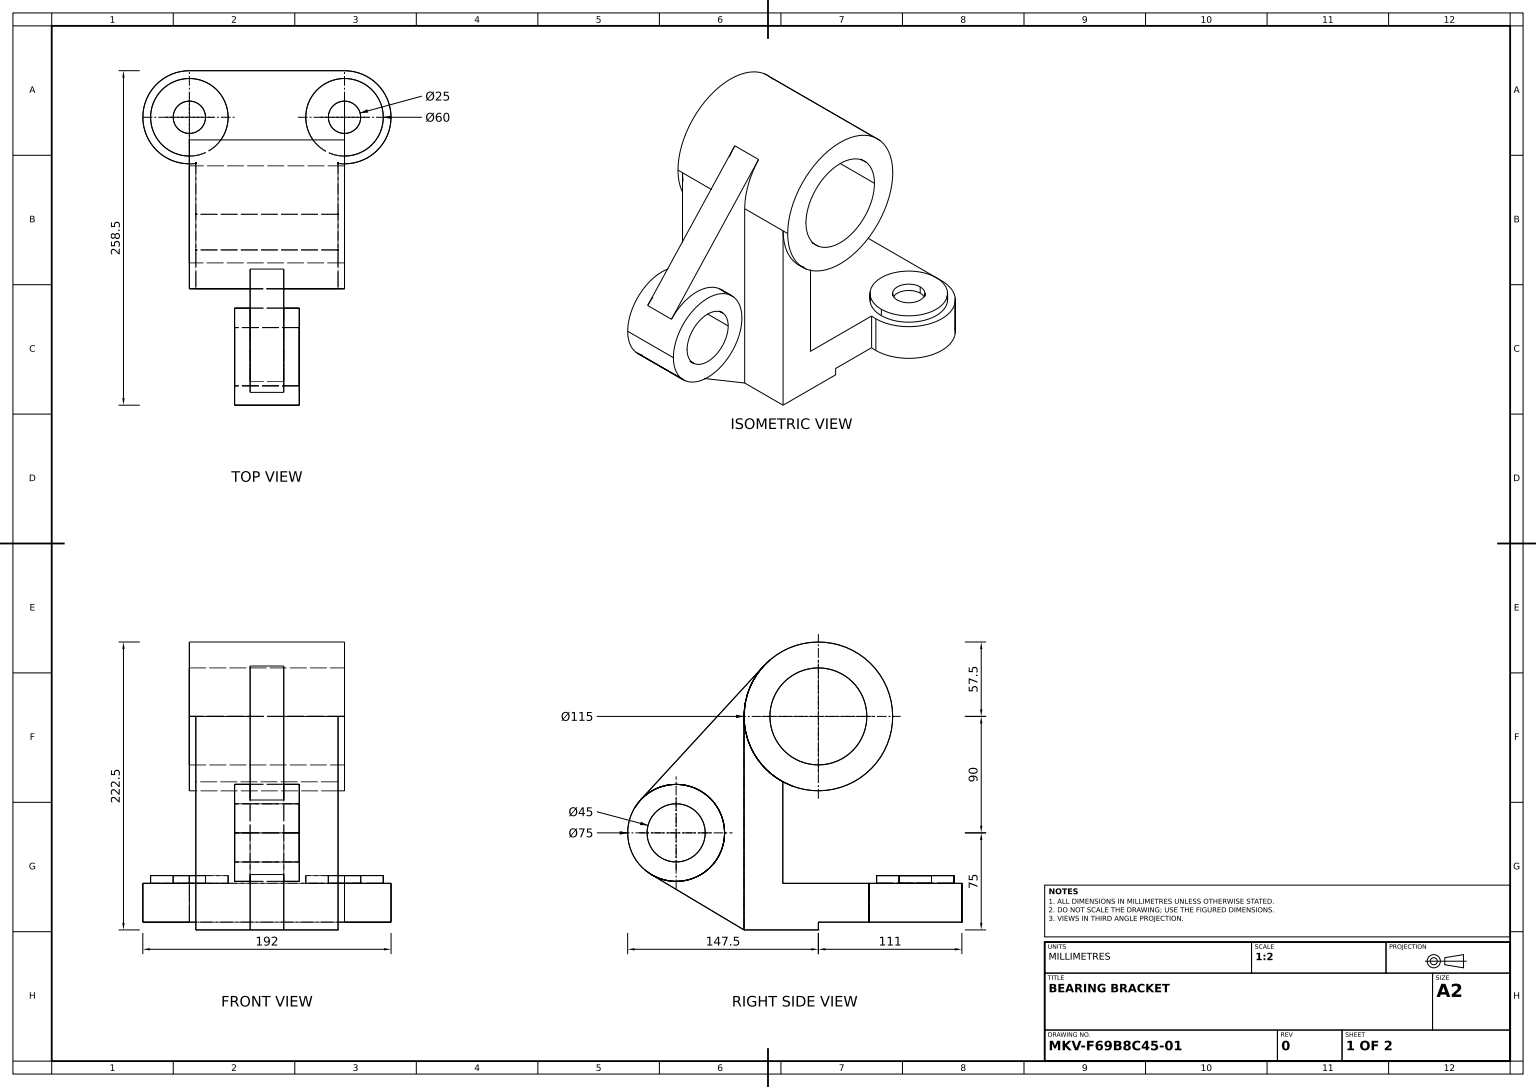
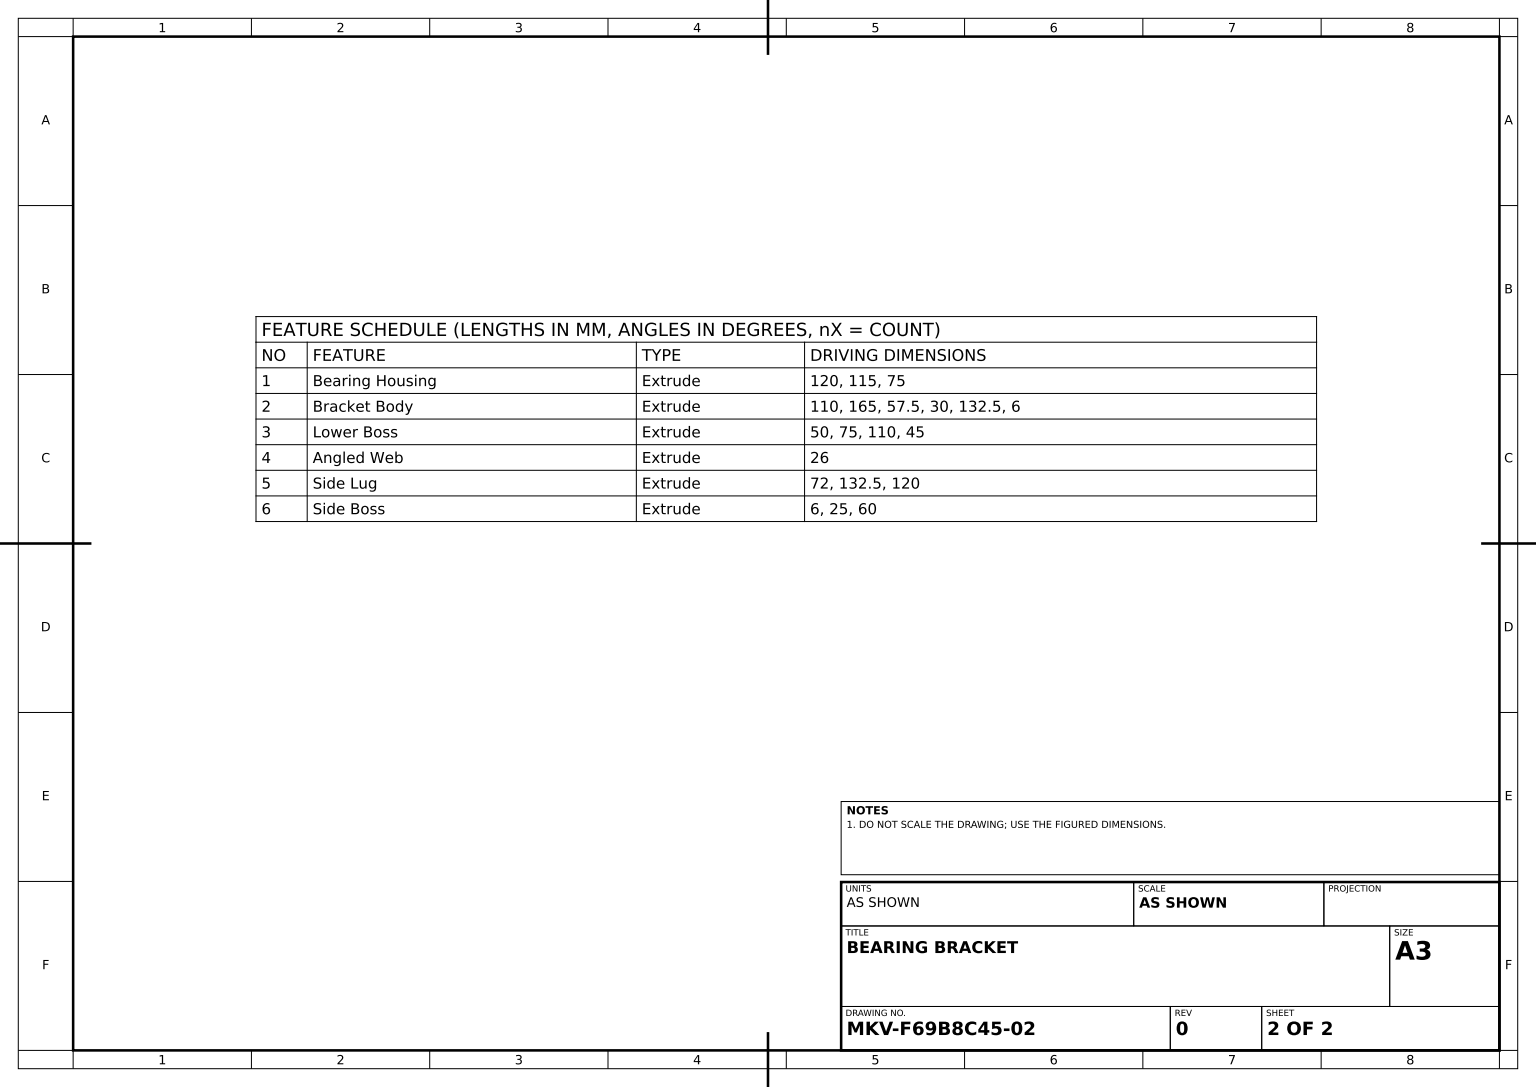
from build123d import *

# Parameters (mm, degrees)
BEARING_HOUSING_SKETCH_R   = 57.5
BEARING_HOUSING_SKETCH_R_2 = 37.5
BEARING_HOUSING_DEPTH      = 60
BRACKET_BODY_DEPTH         = 55
LOWER_BOSS_SKETCH_R        = 37.5
LOWER_BOSS_SKETCH_R_2      = 22.5
LOWER_BOSS_DEPTH           = 25
ANGLED_WEB_DEPTH           = 13
SIDE_LUG_DEPTH             = 30
SIDE_BOSS_SKETCH_R         = 30
SIDE_BOSS_SKETCH_R_2       = 12.5
SIDE_BOSS_DEPTH            = 6


with BuildPart() as part:
    # Bearing Housing Sketch → Bearing Housing (new, symmetric)
    with BuildSketch(Plane(origin=(0, 0, 0), x_dir=(0, 0, -1), z_dir=(1, 0, 0))):
        Circle(BEARING_HOUSING_SKETCH_R)
        Circle(BEARING_HOUSING_SKETCH_R_2, mode=Mode.SUBTRACT)
    extrude(amount=BEARING_HOUSING_DEPTH, both=True)

    # Bracket Body Sketch → Bracket Body (add, symmetric)
    with BuildSketch(Plane(origin=(0, 0, 0), x_dir=(0, 0, -1), z_dir=(1, 0, 0))):
        with BuildLine():
            Line((-57.5, 0), (-57.5, -165))
            Line((-57.5, -165), (0, -165))
            Line((0, -165), (0, -159))
            Line((0, -159), (75, -159))
            Line((75, -159), (75, -129))
            Line((75, -129), (-27.5, -129))
            Line((-27.5, -129), (-27.5, -50.497524692))
            ThreePointArc((-27.5, -50.497524692), (-49.434299833, -29.368350311), (-57.5, 0))
        make_face()
    extrude(amount=BRACKET_BODY_DEPTH, both=True)



with BuildPart() as body_2:
    # Lower Boss Sketch → Lower Boss (new, symmetric)
    with BuildSketch(Plane(origin=(0, 0, 0), x_dir=(0, 0, -1), z_dir=(1, 0, 0))):
        with Locations((-110, -90)):
            Circle(LOWER_BOSS_SKETCH_R)
        with Locations((-110, -90)):
            Circle(LOWER_BOSS_SKETCH_R_2, mode=Mode.SUBTRACT)
    extrude(amount=LOWER_BOSS_DEPTH, both=True)


with BuildPart() as part_1:
    add(part.part)

    add(body_2.part)  # Angled Web merges body 2
    # Angled Web Sketch → Angled Web (add, symmetric)
    with BuildSketch(Plane(origin=(0, 0, 0), x_dir=(0, 0, -1), z_dir=(1, 0, 0))):
        with BuildLine():
            Line((-57.5, 0), (-57.5, -165))
            Line((-57.5, -165), (-129.216934712, -122.201854299))
            ThreePointArc((-129.216934712, -122.201854299), (-72.890500848, -84.60230858), (-137.594286915, -64.606982659))
            Line((-137.594286915, -64.606982659), (-42.311239936, 38.935959922))
            ThreePointArc((-42.311239936, 38.935959922), (-53.568396916, 20.896814394), (-57.5, 0))
        make_face()
    extrude(amount=ANGLED_WEB_DEPTH, both=True)

    # Side Lug Sketch → Side Lug (add)
    with BuildSketch(Plane(origin=(0, -129, 0), x_dir=(1, 0, 0), z_dir=(0, 1, 0))):
        with BuildLine():
            Line((-60, 111), (60, 111))
            ThreePointArc((60, 111), (95.912665801, 72.493920376), (55, 39.34891306))
            Line((55, 39.34891306), (55, -27.5))
            Line((55, -27.5), (-55, -27.5))
            Line((-55, -27.5), (-55, 39.34891306))
            ThreePointArc((-55, 39.34891306), (-95.912665801, 72.493920376), (-60, 111))
        make_face()
    extrude(amount=-SIDE_LUG_DEPTH)

    # Side Boss Sketch → Side Boss (add)
    # profile 1 of 2: a face of its own
    with BuildSketch(Plane(origin=(0, -129, 0), x_dir=(1, 0, 0), z_dir=(0, 1, 0))):
        with Locations(Location((60, 75, 0), (0, 0, 90))):
            Circle(SIDE_BOSS_SKETCH_R)
        with Locations(Location((60, 75, 0), (0, 0, 270))):
            Circle(SIDE_BOSS_SKETCH_R_2, mode=Mode.SUBTRACT)
    # profile 2 of 2: a face of its own
    with BuildSketch(Plane(origin=(0, -129, 0), x_dir=(1, 0, 0), z_dir=(0, 1, 0))):
        with Locations(Location((-60, 75, 0), (0, 0, 90))):
            Circle(SIDE_BOSS_SKETCH_R)
        with Locations(Location((-60, 75, 0), (0, 0, 270))):
            Circle(SIDE_BOSS_SKETCH_R_2, mode=Mode.SUBTRACT)
    extrude(amount=SIDE_BOSS_DEPTH)


solid = part_1.part
